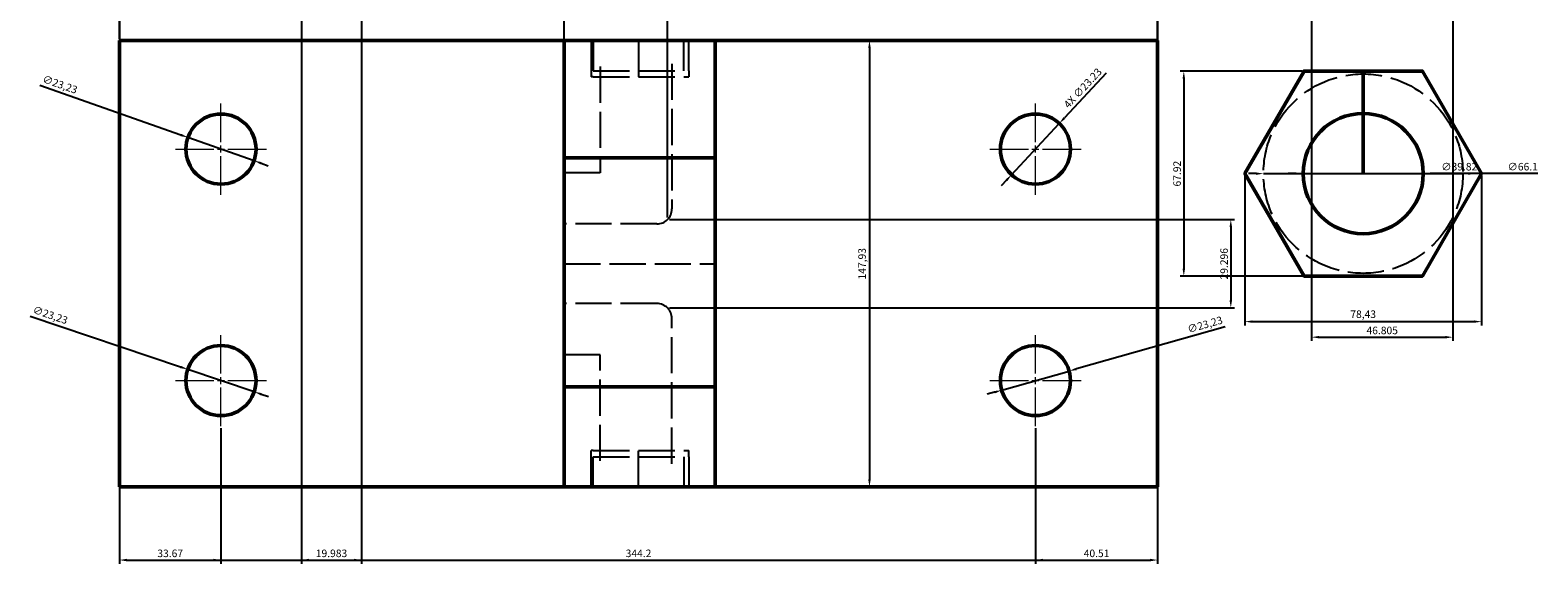
# Model space of a CAD drawing. Units: millimetres. Extents: x 921 to 2648, y 1390 to 2315.
# Tile 1 of 10: x 921 to 1421, y 1705 to 1882. Entities that reach past the tile are written whole.
import ezdxf

# ---------------------------------------------------------------- set-up
doc = ezdxf.new("R2010")
doc.units = ezdxf.units.MM
doc.linetypes.add('ACAD_ISO02W100', pattern=[15, 12, -3])
doc.linetypes.add('CENTER2', pattern=[28.575, 19.05, -3.175, 3.175, -3.175])
for name, color, linetype, lineweight in [('M-CNTR', 1, 'CENTER2', 18), ('M-DIMS', 2, 'Continuous', 25), ('M-HIDN', 4, 'ACAD_ISO02W100', 25), ('M-OUTL', 7, 'Continuous', 50)]:
    doc.layers.add(name, color=color, linetype=linetype, lineweight=lineweight)
doc.styles.get("Standard").update_dxf_attribs({"font": 'arial.ttf'})
doc.dimstyles.new('ISO-25', dxfattribs={"dimtxt": 2.5, "dimasz": 2.5, "dimexe": 1.25, "dimexo": 0.625, "dimtad": 1, "dimtxsty": 'Standard', "dimcen": 2.5, "dimadec": 0, "dimazin": 0, "dimtfac": 1, "dimtmove": 0, "dimatfit": 3, "dimfxl": 1, "dimarcsym": 0})

# ---------------------------------------------------------------- blocks, each defined once
blk = doc.blocks.new('*D13')
at = {"layer": 'Defpoints', "color": 0, "transparency": 16777216}
for p in [(1265.45, 1768.64), (1243.11, 1762.28)]:
    blk.add_point(p, dxfattribs=at)
at = {"layer": 'M-DIMS', "color": 0, "lineweight": -2, "transparency": 16777216}
for p, q in [((1317.12, 1783.33), (1267.86, 1769.32)), ((1243.11, 1762.28), (1265.45, 1768.64)), ((1240.71, 1761.6), (1238.3, 1760.92))]:
    blk.add_line(p, q, dxfattribs=at)
at = {"layer": 'M-DIMS', "color": 0, "transparency": 16777216}
for points in [[(1267.74, 1769.72), (1267.97, 1768.92), (1265.45, 1768.64)], [(1240.59, 1762), (1240.82, 1761.2), (1243.11, 1762.28)]]:
    blk.add_solid(points, dxfattribs=at)
at = {"layer": 'M-DIMS', "color": 0, "transparency": 16777216, "insert": (1310.56, 1783.72), "char_height": 2.5, "attachment_point": 5, "rotation": 15.8769}
blk.add_mtext('∅23,23', dxfattribs=at)
blk = doc.blocks.new('*D14')
at = {"layer": 'Defpoints', "color": 0, "transparency": 16777216}
for p in [(973.33, 1846.05), (995.24, 1838.34)]:
    blk.add_point(p, dxfattribs=at)
at = {"layer": 'M-DIMS', "color": 0, "lineweight": -2, "transparency": 16777216}
for p, q in [((924.24, 1863.35), (970.97, 1846.89)), ((995.24, 1838.34), (973.33, 1846.05)), ((997.59, 1837.5), (999.95, 1836.67))]:
    blk.add_line(p, q, dxfattribs=at)
at = {"layer": 'M-DIMS', "color": 0, "transparency": 16777216}
for points in [[(971.11, 1847.28), (970.83, 1846.49), (973.33, 1846.05)], [(997.73, 1837.9), (997.46, 1837.11), (995.24, 1838.34)]]:
    blk.add_solid(points, dxfattribs=at)
at = {"layer": 'M-DIMS', "color": 0, "transparency": 16777216, "insert": (930.81, 1863.33), "char_height": 2.5, "attachment_point": 5, "rotation": 340.5914}
blk.add_mtext('∅23,23', dxfattribs=at)
blk = doc.blocks.new('*D15')
at = {"layer": 'Defpoints', "color": 0, "transparency": 16777216}
for p in [(973.28, 1769.18), (995.29, 1761.74)]:
    blk.add_point(p, dxfattribs=at)
at = {"layer": 'M-DIMS', "color": 0, "lineweight": -2, "transparency": 16777216}
for p, q in [((921.03, 1786.83), (970.91, 1769.98)), ((995.29, 1761.74), (973.28, 1769.18)), ((997.65, 1760.95), (1000.02, 1760.15))]:
    blk.add_line(p, q, dxfattribs=at)
at = {"layer": 'M-DIMS', "color": 0, "transparency": 16777216}
for points in [[(971.04, 1770.37), (970.78, 1769.58), (973.28, 1769.18)], [(997.79, 1761.34), (997.52, 1760.55), (995.29, 1761.74)]]:
    blk.add_solid(points, dxfattribs=at)
at = {"layer": 'M-DIMS', "color": 0, "transparency": 16777216, "insert": (927.6, 1786.89), "char_height": 2.5, "attachment_point": 5, "rotation": 341.3383}
blk.add_mtext('∅23,23', dxfattribs=at)
blk = doc.blocks.new('*D16')
at = {"layer": 'Defpoints', "color": 0, "transparency": 16777216}
for p in [(1294.79, 1878.16), (1199.26, 1730.23), (1294.79, 1730.23)]:
    blk.add_point(p, dxfattribs=at)
at = {"layer": 'M-DIMS', "color": 0, "lineweight": -2, "transparency": 16777216}
for p, q in [((1294.17, 1878.16), (1198.01, 1878.16)), ((1199.26, 1875.66), (1199.26, 1732.73)), ((1294.17, 1730.23), (1198.01, 1730.23))]:
    blk.add_line(p, q, dxfattribs=at)
at = {"layer": 'M-DIMS', "color": 0, "transparency": 16777216}
for points in [[(1198.84, 1875.66), (1199.67, 1875.66), (1199.26, 1878.16)], [(1198.84, 1732.73), (1199.67, 1732.73), (1199.26, 1730.23)]]:
    blk.add_solid(points, dxfattribs=at)
at = {"layer": 'M-DIMS', "color": 0, "transparency": 16777216, "insert": (1197.13, 1804.19), "char_height": 2.5, "attachment_point": 5, "rotation": 90}
blk.add_mtext('147,93', dxfattribs=at)
blk = doc.blocks.new('*D17')
at = {"layer": 'Defpoints', "color": 0, "transparency": 16777216}
for p in [(1098.08, 1948.7), (950.61, 1892.33), (950.61, 1878.16)]:
    blk.add_point(p, dxfattribs=at)
at = {"layer": 'M-DIMS', "color": 0, "lineweight": -2, "transparency": 16777216}
for p, q in [((1098.08, 1948.07), (1098.08, 1891.08)), ((950.61, 1878.78), (950.61, 1893.58)), ((1095.58, 1892.33), (953.11, 1892.33))]:
    blk.add_line(p, q, dxfattribs=at)
at = {"layer": 'M-DIMS', "color": 0, "transparency": 16777216}
for points in [[(953.11, 1892.74), (953.11, 1891.91), (950.61, 1892.33)], [(1095.58, 1892.74), (1095.58, 1891.91), (1098.08, 1892.33)]]:
    blk.add_solid(points, dxfattribs=at)
at = {"layer": 'M-DIMS', "color": 0, "transparency": 16777216, "insert": (1024.34, 1894.45), "char_height": 2.5, "attachment_point": 5}
blk.add_mtext('147,46', dxfattribs=at)
blk = doc.blocks.new('*D18')
at = {"layer": 'Defpoints', "color": 0, "transparency": 16777216}
for p in [(1148.08, 1948.7), (1294.79, 1892.9), (1294.79, 1878.16)]:
    blk.add_point(p, dxfattribs=at)
at = {"layer": 'M-DIMS', "color": 0, "lineweight": -2, "transparency": 16777216}
for p, q in [((1148.08, 1948.07), (1148.08, 1891.65)), ((1150.58, 1892.9), (1292.29, 1892.9)), ((1294.79, 1878.78), (1294.79, 1894.15))]:
    blk.add_line(p, q, dxfattribs=at)
at = {"layer": 'M-DIMS', "color": 0, "transparency": 16777216}
for points in [[(1150.58, 1893.32), (1150.58, 1892.48), (1148.08, 1892.9)], [(1292.29, 1893.32), (1292.29, 1892.48), (1294.79, 1892.9)]]:
    blk.add_solid(points, dxfattribs=at)
at = {"layer": 'M-DIMS', "color": 0, "transparency": 16777216, "insert": (1221.43, 1895.03), "char_height": 2.5, "attachment_point": 5}
blk.add_mtext('146,72', dxfattribs=at)
blk = doc.blocks.new('*U19')
at = {"layer": 'M-CNTR', "color": 0, "transparency": 16777216}
for p, q in [((0, 2.323), (0, 15.115)), ((-15.115, 0), (-2.323, 0)), ((2.323, 0), (15.115, 0)), ((0, -15.115), (0, -2.323))]:
    blk.add_line(p, q, dxfattribs=at)
at = {"layer": 'M-CNTR', "color": 0, "linetype": 'Continuous', "transparency": 16777216}
for p, q in [((-1.1615, 0), (1.1615, 0)), ((0, -1.1615), (0, 1.1615))]:
    blk.add_line(p, q, dxfattribs=at)
blk = doc.blocks.new('*U20')
at = {"layer": 'M-CNTR', "color": 0, "transparency": 16777216}
for p, q in [((0, 2.323), (0, 15.115)), ((-15.115, 0), (-2.323, 0)), ((2.323, 0), (15.115, 0)), ((0, -15.115), (0, -2.323))]:
    blk.add_line(p, q, dxfattribs=at)
at = {"layer": 'M-CNTR', "color": 0, "linetype": 'Continuous', "transparency": 16777216}
for p, q in [((-1.1615, 0), (1.1615, 0)), ((0, -1.1615), (0, 1.1615))]:
    blk.add_line(p, q, dxfattribs=at)
blk = doc.blocks.new('*U21')
at = {"layer": 'M-CNTR', "color": 0, "transparency": 16777216}
for p, q in [((0, 2.323), (0, 15.115)), ((-15.115, 0), (-2.323, 0)), ((2.323, 0), (15.115, 0)), ((0, -15.115), (0, -2.323))]:
    blk.add_line(p, q, dxfattribs=at)
at = {"layer": 'M-CNTR', "color": 0, "linetype": 'Continuous', "transparency": 16777216}
for p, q in [((-1.1615, 0), (1.1615, 0)), ((0, -1.1615), (0, 1.1615))]:
    blk.add_line(p, q, dxfattribs=at)
blk = doc.blocks.new('*U22')
at = {"layer": 'M-CNTR', "color": 0, "transparency": 16777216}
for p, q in [((0, 2.32), (0, 15.11)), ((-15.11, 0), (-2.32, 0)), ((2.32, 0), (15.11, 0)), ((0, -15.11), (0, -2.32))]:
    blk.add_line(p, q, dxfattribs=at)
at = {"layer": 'M-CNTR', "color": 0, "linetype": 'Continuous', "transparency": 16777216}
for p, q in [((-1.16, 0), (1.16, 0)), ((0, -1.16), (0, 1.16))]:
    blk.add_line(p, q, dxfattribs=at)
blk = doc.blocks.new('*D23')
at = {"layer": 'Defpoints', "color": 0, "transparency": 16777216}
for p in [(1323.71, 1834.06), (1402.14, 1834.06), (1402.14, 1785.01)]:
    blk.add_point(p, dxfattribs=at)
at = {"layer": 'M-DIMS', "color": 0, "lineweight": -2, "transparency": 16777216}
for p, q in [((1323.71, 1833.44), (1323.71, 1783.76)), ((1402.14, 1833.44), (1402.14, 1783.76)), ((1326.21, 1785.01), (1399.64, 1785.01))]:
    blk.add_line(p, q, dxfattribs=at)
at = {"layer": 'M-DIMS', "color": 0, "transparency": 16777216}
for points in [[(1326.21, 1785.43), (1326.21, 1784.6), (1323.71, 1785.01)], [(1399.64, 1785.43), (1399.64, 1784.6), (1402.14, 1785.01)]]:
    blk.add_solid(points, dxfattribs=at)
at = {"layer": 'M-DIMS', "color": 0, "transparency": 16777216, "insert": (1362.92, 1787.14), "char_height": 2.5, "attachment_point": 5}
blk.add_mtext('78,43', dxfattribs=at)
blk = doc.blocks.new('*D47')
at = {"layer": 'Defpoints', "color": 0, "transparency": 16777216}
for p in [(984.28, 1750.35), (950.61, 1730.23), (984.28, 1705.98)]:
    blk.add_point(p, dxfattribs=at)
at = {"layer": 'M-DIMS', "color": 0, "lineweight": -2, "transparency": 16777216}
for p, q in [((984.28, 1749.72), (984.28, 1704.73)), ((950.61, 1729.6), (950.61, 1704.73)), ((953.11, 1705.98), (981.78, 1705.98))]:
    blk.add_line(p, q, dxfattribs=at)
at = {"layer": 'M-DIMS', "color": 0, "transparency": 16777216}
for points in [[(953.11, 1706.4), (953.11, 1705.56), (950.61, 1705.98)], [(981.78, 1706.4), (981.78, 1705.56), (984.28, 1705.98)]]:
    blk.add_solid(points, dxfattribs=at)
at = {"layer": 'M-DIMS', "color": 0, "transparency": 16777216, "insert": (967.45, 1707.88), "char_height": 2.5, "attachment_point": 5}
blk.add_mtext('33.67', dxfattribs=at)
blk = doc.blocks.new('*D48')
at = {"layer": 'Defpoints', "color": 0, "transparency": 16777216}
for p in [(1254.28, 1750.35), (1294.79, 1730.23), (1294.79, 1705.98)]:
    blk.add_point(p, dxfattribs=at)
at = {"layer": 'M-DIMS', "color": 0, "lineweight": -2, "transparency": 16777216}
for p, q in [((1254.28, 1749.72), (1254.28, 1704.73)), ((1294.79, 1729.6), (1294.79, 1704.73)), ((1256.78, 1705.98), (1292.29, 1705.98))]:
    blk.add_line(p, q, dxfattribs=at)
at = {"layer": 'M-DIMS', "color": 0, "transparency": 16777216}
for points in [[(1256.78, 1706.4), (1256.78, 1705.56), (1254.28, 1705.98)], [(1292.29, 1706.4), (1292.29, 1705.56), (1294.79, 1705.98)]]:
    blk.add_solid(points, dxfattribs=at)
at = {"layer": 'M-DIMS', "color": 0, "transparency": 16777216, "insert": (1274.54, 1707.88), "char_height": 2.5, "attachment_point": 5}
blk.add_mtext('40.51', dxfattribs=at)
blk = doc.blocks.new('*D49')
at = {"layer": 'Defpoints', "color": 0, "transparency": 16777216}
for p in [(950.61, 1913.7), (1294.79, 1913.7), (1294.79, 1705.98)]:
    blk.add_point(p, dxfattribs=at)
at = {"layer": 'M-DIMS', "color": 0, "lineweight": -2, "transparency": 16777216}
for p, q in [((950.61, 1913.07), (950.61, 1704.73)), ((1294.79, 1913.07), (1294.79, 1704.73)), ((953.11, 1705.98), (1292.29, 1705.98))]:
    blk.add_line(p, q, dxfattribs=at)
at = {"layer": 'M-DIMS', "color": 0, "transparency": 16777216}
for points in [[(953.11, 1706.4), (953.11, 1705.56), (950.61, 1705.98)], [(1292.29, 1706.4), (1292.29, 1705.56), (1294.79, 1705.98)]]:
    blk.add_solid(points, dxfattribs=at)
at = {"layer": 'M-DIMS', "color": 0, "transparency": 16777216, "insert": (1122.7, 1707.88), "char_height": 2.5, "attachment_point": 5}
blk.add_mtext('344.2', dxfattribs=at)
blk = doc.blocks.new('*D50')
at = {"layer": 'Defpoints', "color": 0, "transparency": 16777216}
for p in [(1132.31, 1818.84), (1132.31, 1789.55), (1319.04, 1789.55)]:
    blk.add_point(p, dxfattribs=at)
at = {"layer": 'M-DIMS', "color": 0, "lineweight": -2, "transparency": 16777216}
for p, q in [((1132.94, 1818.84), (1320.29, 1818.84)), ((1319.04, 1816.34), (1319.04, 1792.05)), ((1132.94, 1789.55), (1320.29, 1789.55))]:
    blk.add_line(p, q, dxfattribs=at)
at = {"layer": 'M-DIMS', "color": 0, "transparency": 16777216}
for points in [[(1318.63, 1816.34), (1319.46, 1816.34), (1319.04, 1818.84)], [(1318.63, 1792.05), (1319.46, 1792.05), (1319.04, 1789.55)]]:
    blk.add_solid(points, dxfattribs=at)
at = {"layer": 'M-DIMS', "color": 0, "transparency": 16777216, "insert": (1317.14, 1804.19), "char_height": 2.5, "attachment_point": 5, "rotation": 90}
blk.add_mtext('29.296', dxfattribs=at)
blk = doc.blocks.new('*D51')
at = {"layer": 'Defpoints', "color": 0, "transparency": 16777216}
for p in [(1132.31, 2203.51), (1098.08, 1817.38), (1132.31, 1818.84)]:
    blk.add_point(p, dxfattribs=at)
at = {"layer": 'M-DIMS', "color": 0, "lineweight": -2, "transparency": 16777216}
for p, q in [((1098.08, 1818), (1098.08, 2204.76)), ((1132.31, 1819.47), (1132.31, 2204.76)), ((1100.58, 2203.51), (1129.81, 2203.51))]:
    blk.add_line(p, q, dxfattribs=at)
at = {"layer": 'M-DIMS', "color": 0, "transparency": 16777216}
for points in [[(1100.58, 2203.93), (1100.58, 2203.1), (1098.08, 2203.51)], [(1129.81, 2203.93), (1129.81, 2203.1), (1132.31, 2203.51)]]:
    blk.add_solid(points, dxfattribs=at)
at = {"layer": 'M-DIMS', "color": 0, "transparency": 16777216, "insert": (1115.19, 2205.42), "char_height": 2.5, "attachment_point": 5}
blk.add_mtext('34.235', dxfattribs=at)
blk = doc.blocks.new('*D53')
at = {"layer": 'Defpoints', "color": 0, "transparency": 16777216}
for p in [(1010.93, 2113.55), (1030.91, 2113.55), (1030.91, 1705.98)]:
    blk.add_point(p, dxfattribs=at)
at = {"layer": 'M-DIMS', "color": 0, "lineweight": -2, "transparency": 16777216}
for p, q in [((1010.93, 2112.93), (1010.93, 1704.73)), ((1030.91, 2112.93), (1030.91, 1704.73)), ((1013.43, 1705.98), (1028.41, 1705.98))]:
    blk.add_line(p, q, dxfattribs=at)
at = {"layer": 'M-DIMS', "color": 0, "transparency": 16777216}
for points in [[(1013.43, 1706.4), (1013.43, 1705.56), (1010.93, 1705.98)], [(1028.41, 1706.4), (1028.41, 1705.56), (1030.91, 1705.98)]]:
    blk.add_solid(points, dxfattribs=at)
at = {"layer": 'M-DIMS', "color": 0, "transparency": 16777216, "insert": (1020.92, 1707.88), "char_height": 2.5, "attachment_point": 5}
blk.add_mtext('19.983', dxfattribs=at)
blk = doc.blocks.new('*D58')
at = {"layer": 'Defpoints', "color": 0, "transparency": 16777216}
for p in [(1345.83, 1891.3), (1392.63, 1891.3), (1392.63, 1779.85)]:
    blk.add_point(p, dxfattribs=at)
at = {"layer": 'M-DIMS', "color": 0, "lineweight": -2, "transparency": 16777216}
for p, q in [((1345.83, 1890.67), (1345.83, 1778.6)), ((1392.63, 1890.67), (1392.63, 1778.6)), ((1348.33, 1779.85), (1390.13, 1779.85))]:
    blk.add_line(p, q, dxfattribs=at)
at = {"layer": 'M-DIMS', "color": 0, "transparency": 16777216}
for points in [[(1348.33, 1780.27), (1348.33, 1779.44), (1345.83, 1779.85)], [(1390.13, 1780.27), (1390.13, 1779.44), (1392.63, 1779.85)]]:
    blk.add_solid(points, dxfattribs=at)
at = {"layer": 'M-DIMS', "color": 0, "transparency": 16777216, "insert": (1369.23, 1781.76), "char_height": 2.5, "attachment_point": 5}
blk.add_mtext('46.805', dxfattribs=at)
blk = doc.blocks.new('*D61')
at = {"layer": 'Defpoints', "color": 0, "transparency": 16777216}
for p in [(1343.32, 1868.02), (1303.46, 1800.1), (1343.32, 1800.1)]:
    blk.add_point(p, dxfattribs=at)
at = {"layer": 'M-DIMS', "color": 0, "lineweight": -2, "transparency": 16777216}
for p, q in [((1342.69, 1868.02), (1302.21, 1868.02)), ((1303.46, 1865.52), (1303.46, 1802.6)), ((1342.69, 1800.1), (1302.21, 1800.1))]:
    blk.add_line(p, q, dxfattribs=at)
at = {"layer": 'M-DIMS', "color": 0, "transparency": 16777216}
for points in [[(1303.04, 1865.52), (1303.88, 1865.52), (1303.46, 1868.02)], [(1303.04, 1802.6), (1303.88, 1802.6), (1303.46, 1800.1)]]:
    blk.add_solid(points, dxfattribs=at)
at = {"layer": 'M-DIMS', "color": 0, "transparency": 16777216, "insert": (1301.56, 1834.06), "char_height": 2.5, "attachment_point": 5, "rotation": 90}
blk.add_mtext('67.92', dxfattribs=at)
blk = doc.blocks.new('*D119')
at = {"layer": 'Defpoints', "color": 0, "transparency": 16777216}
for p in [(1329.87, 1834.06), (1395.97, 1834.06)]:
    blk.add_point(p, dxfattribs=at)
at = {"layer": 'M-DIMS', "color": 0, "lineweight": -2, "transparency": 16777216}
for p, q in [((1327.37, 1834.06), (1324.87, 1834.06)), ((1329.87, 1834.06), (1395.97, 1834.06)), ((1420.8, 1834.06), (1398.47, 1834.06))]:
    blk.add_line(p, q, dxfattribs=at)
at = {"layer": 'M-DIMS', "color": 0, "transparency": 16777216}
for points in [[(1327.37, 1834.48), (1327.37, 1833.65), (1329.87, 1834.06)], [(1398.47, 1834.48), (1398.47, 1833.65), (1395.97, 1834.06)]]:
    blk.add_solid(points, dxfattribs=at)
at = {"layer": 'M-DIMS', "color": 0, "transparency": 16777216, "insert": (1415.81, 1836.04), "char_height": 2.5, "attachment_point": 5, "rotation": 359.9996}
blk.add_mtext('∅66.1', dxfattribs=at)
blk = doc.blocks.new('*D120')
at = {"layer": 'Defpoints', "color": 0, "transparency": 16777216}
for p in [(1343.01, 1834.06), (1382.84, 1834.06)]:
    blk.add_point(p, dxfattribs=at)
at = {"layer": 'M-DIMS', "color": 0, "lineweight": -2, "transparency": 16777216}
for p, q in [((1340.51, 1834.06), (1338.01, 1834.06)), ((1343.01, 1834.06), (1382.84, 1834.06)), ((1400.97, 1834.06), (1385.34, 1834.06))]:
    blk.add_line(p, q, dxfattribs=at)
at = {"layer": 'M-DIMS', "color": 0, "transparency": 16777216}
for points in [[(1340.51, 1834.48), (1340.51, 1833.65), (1343.01, 1834.06)], [(1385.34, 1834.48), (1385.34, 1833.65), (1382.84, 1834.06)]]:
    blk.add_solid(points, dxfattribs=at)
at = {"layer": 'M-DIMS', "color": 0, "transparency": 16777216, "insert": (1394.78, 1836.04), "char_height": 2.5, "attachment_point": 5, "rotation": 359.9993}
blk.add_mtext('∅39.82', dxfattribs=at)
blk = doc.blocks.new('*D125')
at = {"layer": 'Defpoints', "color": 0, "transparency": 16777216}
for p in [(1262.19, 1850.7), (1246.37, 1833.69)]:
    blk.add_point(p, dxfattribs=at)
at = {"layer": 'M-DIMS', "color": 0, "lineweight": -2, "transparency": 16777216}
for p, q in [((1277.68, 1867.35), (1263.9, 1852.53)), ((1246.37, 1833.69), (1262.19, 1850.7)), ((1244.67, 1831.86), (1242.97, 1830.03))]:
    blk.add_line(p, q, dxfattribs=at)
at = {"layer": 'M-DIMS', "color": 0, "transparency": 16777216}
for points in [[(1263.59, 1852.81), (1264.2, 1852.25), (1262.19, 1850.7)], [(1244.36, 1832.14), (1244.97, 1831.58), (1246.37, 1833.69)]]:
    blk.add_solid(points, dxfattribs=at)
at = {"layer": 'M-DIMS', "color": 0, "transparency": 16777216, "insert": (1270.2, 1862.2), "char_height": 2.5, "attachment_point": 5, "rotation": 47.0707}
blk.add_mtext('4X ∅23.23', dxfattribs=at)

msp = doc.modelspace()

# ---------------------------------------------------------------- linework, layer by layer
at = {"layer": 'M-HIDN'}
for p, q in [((1106.9781, 1878.159), (1106.9781, 1868.159)), ((1122.7038, 1878.159), (1107.7038, 1878.159)), ((1107.7038, 1878.159), (1107.7038, 1868.159)), ((1122.7038, 1878.159), (1122.7038, 1866.1215)), ((1137.7038, 1868.159), (1137.7038, 1878.159)), ((1139.3365, 1868.159), (1139.3365, 1878.159)), ((1109.9508, 1869.5673), (1109.9508, 1834.3454)), ((1133.7752, 1870.4989), (1133.7752, 1822.3777)), ((1106.9781, 1868.159), (1106.9781, 1866.1215)), ((1107.7038, 1866.1215), (1106.9781, 1866.1215)), ((1107.7038, 1868.159), (1137.7038, 1868.159)), ((1107.7038, 1866.1215), (1137.7038, 1866.1215)), ((1137.7038, 1866.1215), (1139.3365, 1866.1215)), ((1139.3365, 1868.159), (1139.3365, 1866.1215)), ((1109.9508, 1834.3454), (1098.0755, 1834.3454)), ((1128.7752, 1817.3777), (1098.0755, 1817.3777)), ((1098.0755, 1804.1943), (1148.0755, 1804.1943)), ((1128.7752, 1791.0108), (1098.0755, 1791.0108)), ((1133.7752, 1737.8896), (1133.7752, 1786.0108)), ((1109.9508, 1774.0431), (1098.0755, 1774.0431)), ((1109.9508, 1738.8212), (1109.9508, 1774.0431)), ((1106.9781, 1740.2295), (1106.9781, 1742.267)), ((1107.7038, 1742.267), (1106.9781, 1742.267)), ((1106.9781, 1730.2295), (1106.9781, 1740.2295)), ((1107.7038, 1742.267), (1137.7038, 1742.267)), ((1107.7038, 1730.2295), (1107.7038, 1740.2295)), ((1107.7038, 1740.2295), (1137.7038, 1740.2295)), ((1122.7038, 1730.2295), (1122.7038, 1742.267)), ((1137.7038, 1742.267), (1139.3365, 1742.267)), ((1137.7038, 1740.2295), (1137.7038, 1730.2295)), ((1139.3365, 1740.2295), (1139.3365, 1742.267)), ((1139.3365, 1740.2295), (1139.3365, 1730.2295)), ((1122.7038, 1730.2295), (1107.7038, 1730.2295))]:
    msp.add_line(p, q, dxfattribs=at)
msp.add_circle((1362.9248, 1834.0642), 33.0501, dxfattribs=at)
for centre, start, end in [((1128.7752, 1822.3777), 270, 0), ((1128.7752, 1786.0108), 0, 90)]:
    msp.add_arc(centre, 5, start, end, dxfattribs=at)
at = {"layer": 'M-OUTL'}
for p, q in [((950.6135, 1878.159), (1294.7941, 1878.159)), ((950.6135, 1878.159), (950.6135, 1730.2295)), ((1098.0755, 1878.159), (1098.0755, 1730.2295)), ((1148.0755, 1878.159), (1148.0755, 1730.2295)), ((1294.7941, 1878.159), (1294.7941, 1859.6497)), ((1362.9248, 1868.0248), (1362.9248, 1834.0642)), ((1294.7941, 1859.6497), (1294.7941, 1730.2295)), ((1098.0755, 1839.327), (1148.0755, 1839.327)), ((1098.0755, 1763.3619), (1148.0755, 1763.3619)), ((950.6135, 1730.2295), (1294.7941, 1730.2295))]:
    msp.add_line(p, q, dxfattribs=at)
msp.add_lwpolyline([(1402.1391, 1834.0642), (1382.532, 1868.0248), (1343.3176, 1868.0248), (1323.7105, 1834.0642), (1343.3176, 1800.1036), (1382.532, 1800.1036)], close=True, dxfattribs=at)
for centre, radius in [((984.2815, 1842.1949), 11.615), ((1254.2815, 1842.1949), 11.615), ((1362.9248, 1834.0642), 19.9112), ((984.2815, 1765.4616), 11.615), ((1254.2815, 1765.4616), 11.6137)]:
    msp.add_circle(centre, radius, dxfattribs=at)

# ---------------------------------------------------------------- block references
at = {"layer": 'M-CNTR'}
for name, p in [('*U19', (984.2815, 1842.1949)), ('*U21', (1254.2815, 1842.1949)), ('*U20', (984.2815, 1765.4616)), ('*U22', (1254.2815, 1765.4616))]:
    msp.add_blockref(name, p, dxfattribs=at)

# ---------------------------------------------------------------- dimensions: what is measured, and where the dimension line sits
at = {"layer": 'M-DIMS'}
for base, p1, p2, override, picture, middle in [((1132.3108, 2203.5149), (1098.0755, 1817.3777), (1132.3108, 1818.8422), {"dimdec": 3, "dimlfac": 1, "dimrnd": 0, "dimzin": 0, "dimdsep": 46, "dimlunit": 2}, '*D51', (1115.1932, 2205.4172)), ((1030.90998, 1705.9795), (1010.92747, 2113.5505), (1030.90998, 2113.5505), {"dimdec": 3, "dimlfac": 1, "dimrnd": 0, "dimzin": 0, "dimdsep": 46, "dimlunit": 2}, '*D53', (1020.91873, 1707.88179)), ((950.6135, 1892.3265), (1098.0755, 1948.699), (950.6135, 1878.159), {"dimclrd": 0, "dimclre": 0, "dimclrt": 0}, '*D17', (1024.3445, 1894.4539)), ((1294.7941, 1892.9016), (1148.0755, 1948.699), (1294.7941, 1878.159), {"dimclrd": 0, "dimclre": 0, "dimclrt": 0}, '*D18', (1221.4348, 1895.029)), ((1294.7941, 1705.9795), (950.6135, 1913.699), (1294.7941, 1913.699), {"dimdec": 1, "dimlfac": 1, "dimrnd": 0, "dimzin": 0, "dimdsep": 46, "dimlunit": 2}, '*D49', (1122.7038, 1707.8818)), ((1392.6304, 1779.8536), (1345.8257, 1891.2986), (1392.6304, 1891.2986), {"dimdec": 3, "dimlfac": 1, "dimrnd": 0, "dimzin": 0, "dimdsep": 46, "dimlunit": 2}, '*D58', (1369.2281, 1781.7551)), ((1402.1391, 1785.012), (1323.7105, 1834.0642), (1402.1391, 1834.0642), {"dimclrd": 0, "dimclre": 0, "dimclrt": 0}, '*D23', (1362.9248, 1787.1394)), ((984.2815, 1705.9795), (950.6135, 1730.2295), (984.2815, 1750.3466), {"dimdec": 2, "dimlfac": 1, "dimrnd": 0, "dimzin": 0, "dimdsep": 46, "dimlunit": 2}, '*D47', (967.4475, 1707.8818)), ((1294.7941, 1705.9795), (1254.2815, 1750.3479), (1294.7941, 1730.2295), {"dimdec": 2, "dimlfac": 1, "dimrnd": 0, "dimzin": 0, "dimdsep": 46, "dimlunit": 2}, '*D48', (1274.5378, 1707.8809))]:
    dim = msp.add_linear_dim(base=base, p1=p1, p2=p2, dimstyle='ISO-25', override=override, dxfattribs=at)
    dim.commit()
    dim.dimension.update_dxf_attribs({"geometry": picture, "text_midpoint": middle})
for base, p1, p2, override, picture, middle in [((1199.2567, 1730.2295), (1294.7941, 1878.159), (1294.7941, 1730.2295), {"dimclrd": 0, "dimclre": 0, "dimclrt": 0}, '*D16', (1197.1293, 1804.1943)), ((1303.4605, 1800.1036), (1343.3176, 1868.0248), (1343.3176, 1800.1036), {"dimdec": 2, "dimlfac": 1, "dimrnd": 0, "dimzin": 0, "dimdsep": 46, "dimlunit": 2}, '*D61', (1301.559, 1834.0642)), ((1319.0441, 1789.5463), (1132.3108, 1818.8422), (1132.3108, 1789.5463), {"dimdec": 3, "dimlfac": 1, "dimrnd": 0, "dimzin": 0, "dimdsep": 46, "dimlunit": 2}, '*D50', (1317.1427, 1804.1943))]:
    dim = msp.add_linear_dim(base=base, p1=p1, p2=p2, angle=90, dimstyle='ISO-25', override=override, dxfattribs=at)
    dim.commit()
    dim.dimension.update_dxf_attribs({"geometry": picture, "text_midpoint": middle})
for p1, p2, override, picture, middle in [((995.2364, 1838.3352), (973.3265, 1846.0546), {"dimclrd": 0, "dimclre": 0, "dimclrt": 0}, '*D14', (930.0911, 1861.2875)), ((1329.8746, 1834.0645), (1395.9749, 1834.064), {"dimdec": 1, "dimlfac": 1, "dimrnd": 0, "dimzin": 0, "dimdsep": 46, "dimlunit": 2}, '*D119', (1415.805, 1834.0639)), ((1343.0136, 1834.0645), (1382.8359, 1834.064), {"dimdec": 2, "dimlfac": 1, "dimrnd": 0, "dimzin": 0, "dimdsep": 46, "dimlunit": 2}, '*D120', (1394.7826, 1834.0639)), ((995.2858, 1761.745), (973.2772, 1769.1781), {"dimclrd": 0, "dimclre": 0, "dimclrt": 0}, '*D15', (926.903, 1784.8404)), ((1243.1108, 1762.2844), (1265.4521, 1768.6387), {"dimclrd": 0, "dimclre": 0, "dimclrt": 0}, '*D13', (1311.1554, 1781.6378))]:
    dim = msp.add_diameter_dim_2p(p1=p1, p2=p2, dimstyle='ISO-25', override=override, dxfattribs=at)
    dim.commit()
    dim.dimension.update_dxf_attribs({"geometry": picture, "text_midpoint": middle, "dimtype": 163})
dim = msp.add_diameter_dim_2p(p1=(1246.3706, 1833.6905), p2=(1262.1924, 1850.6993), text='4X <>', dimstyle='ISO-25', override={"dimdec": 2, "dimlfac": 1, "dimrnd": 0, "dimzin": 0, "dimdsep": 46, "dimlunit": 2}, dxfattribs=at)
dim.commit()
dim.dimension.update_dxf_attribs({"geometry": '*D125', "text_midpoint": (1271.6411, 1860.8569)})

doc.saveas('drawing.dxf')
